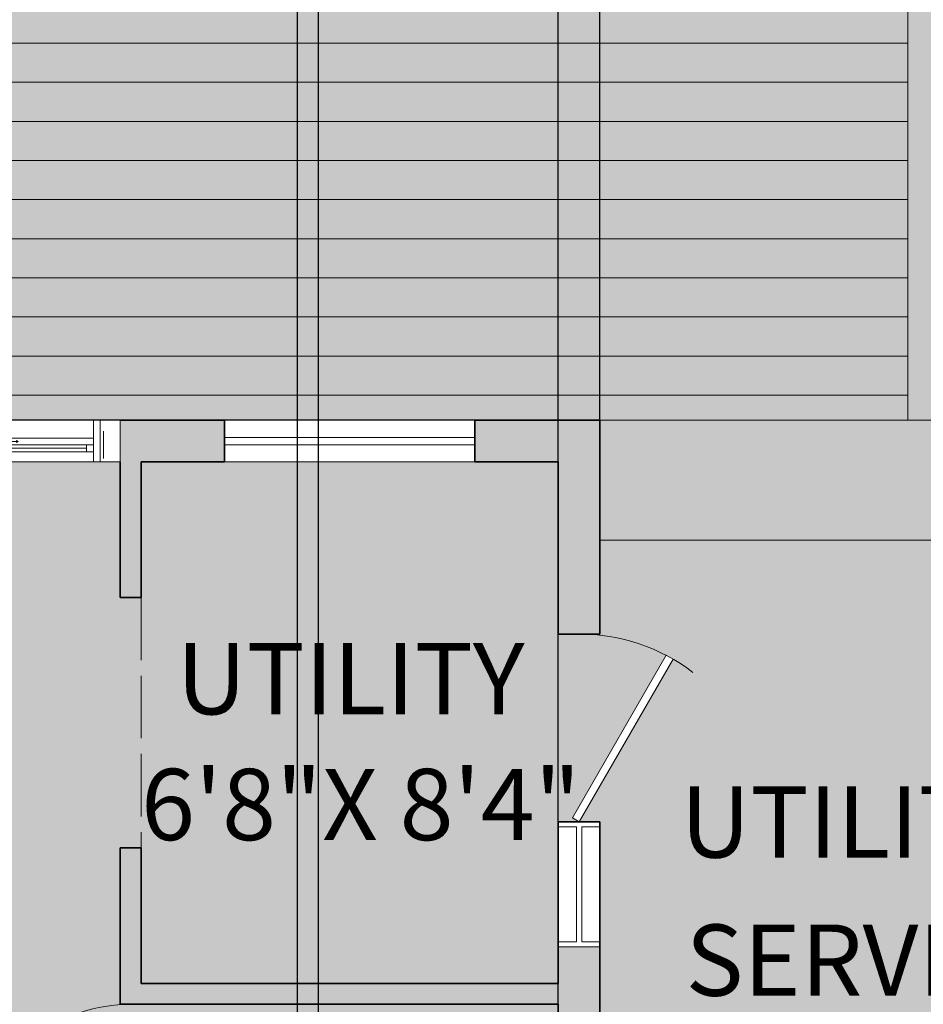
# Model space of a CAD drawing. Units: inches. Extents: x 1704 to 6393, y -157 to 1172.
# Tile 90 of 122: x 2494 to 2667, y 783 to 972. Entities that reach past the tile are written whole.
import ezdxf

# ---------------------------------------------------------------- set-up
doc = ezdxf.new("R2010")
doc.units = ezdxf.units.IN
doc.header["$MEASUREMENT"] = 0
doc.linetypes.add('ACAD_ISO02W100', pattern=[15, 12, -3])
for name, color, linetype, lineweight in [('A-ANNO-DIMS', 7, 'Continuous', 13), ('A-AREA-IDEN', 7, 'Continuous', 18), ('A-WALL-OVHD', 8, 'ACAD_ISO02W100', 13), ('A-WALL-PATT', 7, 'Continuous', 13), ('DOORS', 160, 'Continuous', 18), ('GLASS PANEL FASADE', 4, 'Continuous', 18), ('L-DECK-PLNK-PATT', 250, 'Continuous', 13), ('L-HRDS', 8, 'Continuous', 18), ('WALLS', 7, 'Continuous', 35), ('WINDOWS', 2, 'Continuous', 18)]:
    doc.layers.add(name, color=color, linetype=linetype, lineweight=lineweight)
for name, color, linetype, lineweight, true_color in [('A-FLOR-PATT', 7, 'Continuous', 13, 0xf2f2f2), ('L-DECK-PATT', 35, 'Continuous', 13, 0xa6725b), ('L-HRDS-PATT', 9, 'Continuous', 13, 0xc5c1ba)]:
    doc.layers.add(name, color=color, linetype=linetype, lineweight=lineweight, true_color=true_color)
doc.styles.get("Standard").update_dxf_attribs({"font": 'arial.ttf'})
doc.dimstyles.get("Standard").update_dxf_attribs({"dimtxt": 6, "dimasz": 2, "dimexe": 0.18, "dimexo": 0.0625, "dimgap": 0.09, "dimtad": 0, "dimtih": 1, "dimtoh": 1, "dimdec": 1, "dimzin": 0, "dimdsep": 46, "dimlunit": 3, "dimtxsty": 'Standard', "dimblk": 'ARCHTICK', "dimcen": 0.09, "dimadec": 0, "dimazin": 0, "dimtfac": 1, "dimtdec": 1, "dimtofl": 0, "dimtmove": 0, "dimatfit": 3, "dimfxl": 1, "dimtolj": 1, "dimtzin": 0, "dimarcsym": 0})

# ---------------------------------------------------------------- blocks, each defined once
blk = doc.blocks.new('Door - Left Hung 36 in.')
blk.add_lwpolyline([(0.75, -1.3), (0, 0), (31.18, 18), (31.93, 16.7)], close=True)
blk.add_arc((0, 0), 36, 0, 37.3101)
blk = doc.blocks.new('WIN-SLIDER-48')
for p, q in [((3.83, 8), (0, 8)), ((5.13, 8), (42.87, 8)), ((44.17, 8), (48, 8)), ((3.18, 5.86), (3.18, 0.65)), ((44.82, 5.86), (44.82, 0.65)), ((6.43, 4.55), (22.7, 4.55)), ((6.43, 3.9), (22.7, 3.9)), ((24, 4.55), (42.87, 4.55)), ((25.3, 3.9), (28.1, 3.9)), ((24, 1.95), (5.13, 1.95)), ((6.43, 3.25), (22.7, 3.25)), ((22.7, 2.6), (19.9, 2.6)), ((25.3, 3.25), (41.56, 3.25)), ((25.3, 2.6), (41.56, 2.6)), ((25.3, 1.95), (41.56, 1.95)), ((3.83, 0), (0, 0)), ((5.13, 0), (42.87, 0)), ((44.17, 0), (48, 0))]:
    blk.add_line(p, q)
for points in [[(5.13, 0), (3.83, 0), (3.83, 8), (5.13, 8)], [(42.87, 0), (44.17, 0), (44.17, 8), (42.87, 8)], [(5.13, 3.25), (6.43, 3.25), (6.43, 4.55), (5.13, 4.55)], [(22.7, 3.25), (24, 3.25), (24, 4.55), (22.7, 4.55)], [(28.43, 3.9), (28.1, 4.1), (28.1, 3.71)], [(19.57, 2.6), (19.9, 2.8), (19.9, 2.41)], [(24, 1.95), (25.3, 1.95), (25.3, 3.25), (24, 3.25)], [(41.56, 1.95), (42.87, 1.95), (42.87, 3.25), (41.56, 3.25)]]:
    blk.add_lwpolyline(points, close=True)
blk = doc.blocks.new('WIN-VENT-24')
for p, q in [((0, 0), (0, 24)), ((0, 24), (8, 24)), ((0, 23), (3.5, 23)), ((3.5, 23), (3.5, 1)), ((4.5, 23), (8, 23)), ((4.5, 23), (4.5, 1)), ((8, 24), (8, 0)), ((3.5, 1), (0, 1)), ((8, 1), (4.5, 1)), ((8, 0), (0, 0))]:
    blk.add_line(p, q)
blk = doc.blocks.new('_ArchTick')
at = {"color": 0, "linetype": 'ByBlock', "const_width": 0.15}
blk.add_lwpolyline([(-0.5, -0.5), (0.5, 0.5)], dxfattribs=at)
blk = doc.blocks.new('*D92')
at = {"layer": 'A-ANNO-DIMS', "color": 0, "lineweight": -2, "transparency": 16777216}
for p, q in [((2073.35, 895.28), (2073.35, 1105.29)), ((2073.35, 1105.11), (2332.66, 1105.11)), ((2605.35, 1105.11), (2346.04, 1105.11)), ((2605.35, 895.28), (2605.35, 1105.29))]:
    blk.add_line(p, q, dxfattribs=at)
at = {"layer": 'Defpoints', "color": 0, "lineweight": -3, "transparency": 16777216}
for p in [(2605.35, 1105.11), (2073.35, 895.21), (2605.35, 895.21)]:
    blk.add_point(p, dxfattribs=at)
at = {"layer": 'A-ANNO-DIMS', "color": 0, "lineweight": -2, "transparency": 16777216, "xscale": 2, "yscale": 2, "zscale": 2, "rotation": 180}
blk.add_blockref('_ArchTick', (2073.35, 1105.11), dxfattribs=at)
at = {"layer": 'A-ANNO-DIMS', "color": 0, "lineweight": -2, "transparency": 16777216, "xscale": 2, "yscale": 2, "zscale": 2}
blk.add_blockref('_ArchTick', (2605.35, 1105.11), dxfattribs=at)
at = {"layer": 'A-ANNO-DIMS', "color": 0, "transparency": 16777216, "insert": (2339.35, 1105.11), "char_height": 6, "attachment_point": 5}
blk.add_mtext('\\A1;532', dxfattribs=at)
blk = doc.blocks.new('*D93')
at = {"layer": 'A-ANNO-DIMS', "color": 0, "lineweight": -2, "transparency": 16777216}
for p, q in [((2605.29, 895.21), (1829.7, 895.21)), ((1829.88, 895.21), (1829.88, 495.87)), ((1829.88, 90.21), (1829.88, 489.56)), ((2605.29, 90.21), (1829.7, 90.21))]:
    blk.add_line(p, q, dxfattribs=at)
at = {"layer": 'Defpoints', "color": 0, "lineweight": -3, "transparency": 16777216}
for p in [(2605.35, 895.21), (1829.88, 90.21), (2605.35, 90.21)]:
    blk.add_point(p, dxfattribs=at)
at = {"layer": 'A-ANNO-DIMS', "color": 0, "lineweight": -2, "transparency": 16777216, "xscale": 2, "yscale": 2, "zscale": 2}
for p, rotation in [((1829.88, 895.21), 90), ((1829.88, 90.21), 270)]:
    blk.add_blockref('_ArchTick', p, dxfattribs=dict(at, rotation=rotation))
at = {"layer": 'A-ANNO-DIMS', "color": 0, "transparency": 16777216, "insert": (1829.88, 492.71), "char_height": 6, "attachment_point": 5}
blk.add_mtext('\\A1;805', dxfattribs=at)
blk = doc.blocks.new('*D95')
at = {"layer": 'A-ANNO-DIMS', "color": 0, "lineweight": -2, "transparency": 16777216}
for p, q in [((2605.35, 895.28), (2605.35, 1105.29)), ((2605.35, 1105.11), (2657.91, 1105.11)), ((2723.35, 1105.11), (2670.79, 1105.11)), ((2723.35, 895.28), (2723.35, 1105.29))]:
    blk.add_line(p, q, dxfattribs=at)
at = {"layer": 'Defpoints', "color": 0, "lineweight": -3, "transparency": 16777216}
for p in [(2723.35, 1105.11), (2605.35, 895.21), (2723.35, 895.21)]:
    blk.add_point(p, dxfattribs=at)
at = {"layer": 'A-ANNO-DIMS', "color": 0, "lineweight": -2, "transparency": 16777216, "xscale": 2, "yscale": 2, "zscale": 2, "rotation": 180}
blk.add_blockref('_ArchTick', (2605.35, 1105.11), dxfattribs=at)
at = {"layer": 'A-ANNO-DIMS', "color": 0, "lineweight": -2, "transparency": 16777216, "xscale": 2, "yscale": 2, "zscale": 2}
blk.add_blockref('_ArchTick', (2723.35, 1105.11), dxfattribs=at)
at = {"layer": 'A-ANNO-DIMS', "color": 0, "transparency": 16777216, "insert": (2664.35, 1105.11), "char_height": 6, "attachment_point": 5}
blk.add_mtext('\\A1;118', dxfattribs=at)
blk = doc.blocks.new('*D102')
at = {"layer": 'A-ANNO-DIMS', "color": 0, "lineweight": -2, "transparency": 16777216}
for p, q in [((2367.74, 711.28), (2367.74, 1105.29)), ((2367.74, 1105.11), (2447.61, 1105.11)), ((2547.35, 1105.11), (2467.47, 1105.11)), ((2547.35, 711.28), (2547.35, 1105.29))]:
    blk.add_line(p, q, dxfattribs=at)
at = {"layer": 'Defpoints', "color": 0, "lineweight": -3, "transparency": 16777216}
for p in [(2547.35, 1105.11), (2367.74, 711.21), (2547.35, 711.21)]:
    blk.add_point(p, dxfattribs=at)
at = {"layer": 'A-ANNO-DIMS', "color": 0, "lineweight": -2, "transparency": 16777216, "xscale": 2, "yscale": 2, "zscale": 2, "rotation": 180}
blk.add_blockref('_ArchTick', (2367.74, 1105.11), dxfattribs=at)
at = {"layer": 'A-ANNO-DIMS', "color": 0, "lineweight": -2, "transparency": 16777216, "xscale": 2, "yscale": 2, "zscale": 2}
blk.add_blockref('_ArchTick', (2547.35, 1105.11), dxfattribs=at)
at = {"layer": 'A-ANNO-DIMS', "color": 0, "transparency": 16777216, "insert": (2457.54, 1105.11), "char_height": 6, "attachment_point": 5}
blk.add_mtext('\\A1;179.6', dxfattribs=at)
blk = doc.blocks.new('*D103')
at = {"layer": 'A-ANNO-DIMS', "color": 0, "lineweight": -2, "transparency": 16777216}
for p, q in [((2551.35, 711.28), (2551.35, 1105.29)), ((2551.35, 1105.11), (2569.84, 1105.11)), ((2597.35, 1105.11), (2578.85, 1105.11)), ((2597.35, 711.28), (2597.35, 1105.29))]:
    blk.add_line(p, q, dxfattribs=at)
at = {"layer": 'Defpoints', "color": 0, "lineweight": -3, "transparency": 16777216}
for p in [(2597.35, 1105.11), (2551.35, 711.21), (2597.35, 711.21)]:
    blk.add_point(p, dxfattribs=at)
at = {"layer": 'A-ANNO-DIMS', "color": 0, "lineweight": -2, "transparency": 16777216, "xscale": 2, "yscale": 2, "zscale": 2, "rotation": 180}
blk.add_blockref('_ArchTick', (2551.35, 1105.11), dxfattribs=at)
at = {"layer": 'A-ANNO-DIMS', "color": 0, "lineweight": -2, "transparency": 16777216, "xscale": 2, "yscale": 2, "zscale": 2}
blk.add_blockref('_ArchTick', (2597.35, 1105.11), dxfattribs=at)
at = {"layer": 'A-ANNO-DIMS', "color": 0, "transparency": 16777216, "insert": (2574.35, 1105.11), "char_height": 6, "attachment_point": 5}
blk.add_mtext('\\A1;46', dxfattribs=at)

msp = doc.modelspace()

# ---------------------------------------------------------------- hatches: boundary and pattern name
at = {"layer": 'A-FLOR-PATT', "transparency": 33554528}
h = msp.add_hatch(color=256, dxfattribs=at)
h.dxf.hatch_style = 1
h.paths.add_polyline_path([(2517.349, 861.213), (2513.349, 861.213), (2513.349, 887.213), (2509.516, 887.213), (2508.215, 887.213), (2470.482, 887.213), (2469.181, 887.213), (2465.349, 887.213), (2333.349, 887.213), (2333.349, 863.213), (2325.349, 863.213), (2325.349, 763.213), (2365.349, 763.213), (2365.349, 719.213), (2513.349, 719.213), (2513.349, 753.213), (2515.349, 753.213), (2500.349, 779.194), (2501.431, 779.819), (2501.444, 779.796, -0.1041754), (2513.349, 783.146), (2513.349, 813.213), (2517.349, 813.213)])
h.paths.add_polyline_path([(2597.349, 818.213), (2601.349, 818.213), (2600.05, 818.963), (2618.034, 850.113, 0.1210664), (2601.349, 854.213), (2597.349, 854.213), (2597.349, 887.213), (2581.349, 887.213), (2533.349, 887.213), (2517.349, 887.213), (2517.349, 861.213), (2517.349, 813.213), (2517.349, 787.213), (2597.349, 787.213)])
h.paths.add_polyline_path([(2597.349, 783.213), (2517.349, 783.213), (2515.349, 783.213, 0.1210664), (2501.444, 779.796), (2516.792, 753.213), (2517.349, 753.213), (2517.349, 719.213), (2597.349, 719.213)])
at = {"layer": 'A-WALL-PATT', "transparency": 33554643}
h = msp.add_hatch(color=256, dxfattribs=at)
h.dxf.hatch_style = 1
h.paths.add_polyline_path([(2167.349, 895.213), (2073.349, 895.213), (2073.349, 887.213), (2081.349, 887.213), (2167.349, 887.213)])
h.paths.add_polyline_path([(2465.349, 895.213), (2273.349, 895.213), (2273.349, 903.213), (2263.349, 903.213), (2263.349, 895.213), (2263.349, 887.213), (2325.349, 887.213), (2325.349, 863.213), (2333.349, 863.213), (2333.349, 887.213), (2465.349, 887.213)])
h.paths.add_polyline_path([(2533.349, 895.213), (2513.349, 895.213), (2513.349, 887.213), (2513.349, 861.213), (2517.349, 861.213), (2517.349, 887.213), (2533.349, 887.213)])
h.paths.add_polyline_path([(2605.349, 895.213), (2581.349, 895.213), (2581.349, 887.213), (2597.349, 887.213), (2597.349, 854.213), (2605.349, 854.213)])
h.paths.add_polyline_path([(2605.349, 752.213), (2629.349, 752.213), (2629.349, 716.213), (2605.349, 716.213), (2605.349, 712.213), (2719.349, 712.213), (2719.349, 716.213), (2631.349, 716.213), (2631.349, 754.213), (2605.349, 754.213), (2605.349, 794.213), (2597.349, 794.213), (2597.349, 787.213), (2517.349, 787.213), (2517.349, 813.213), (2513.349, 813.213), (2513.349, 783.213), (2517.349, 783.213), (2597.349, 783.213), (2597.349, 719.213), (2517.349, 719.213), (2517.349, 753.213), (2513.349, 753.213), (2513.349, 719.213), (2365.349, 719.213), (2365.349, 763.213), (2325.349, 763.213), (2325.349, 755.213), (2357.349, 755.213), (2357.349, 719.213), (2325.349, 719.213), (2325.349, 711.213), (2547.349, 711.213), (2547.349, 615.213), (2449.349, 615.213), (2449.349, 607.213), (2514.349, 607.213), (2514.349, 546.213), (2439.349, 546.213), (2425.349, 546.213), (2425.349, 607.213), (2425.349, 615.213), (2350.349, 615.213), (2350.349, 589.713), (2358.349, 589.713), (2358.349, 610.213), (2420.349, 610.213), (2420.349, 545.213), (2358.349, 545.213), (2358.349, 565.713), (2350.349, 565.713), (2350.349, 538.213), (2469.349, 538.213), (2469.349, 459.213), (2469.349, 372.213), (2423.349, 372.213), (2423.349, 364.213), (2473.349, 364.213), (2473.349, 318.213), (2477.349, 318.213), (2477.349, 364.213), (2547.349, 364.213), (2547.349, 352.213), (2549.349, 352.213), (2549.349, 364.213), (2597.349, 364.213), (2597.349, 328.213), (2549.349, 328.213), (2547.349, 328.213), (2547.349, 326.213), (2549.349, 326.213), (2597.349, 326.213), (2605.349, 326.213), (2605.349, 377.057), (2597.349, 377.057), (2597.349, 372.213), (2477.349, 372.213), (2477.349, 451.213), (2597.349, 451.213), (2605.349, 451.213), (2605.349, 459.213), (2597.349, 459.213), (2477.349, 459.213), (2477.349, 538.213), (2597.349, 538.213), (2597.349, 495.213), (2605.349, 495.213), (2605.349, 512.213), (2631.349, 512.213), (2631.349, 568.213), (2605.349, 568.213), (2605.349, 577.213), (2597.349, 577.213), (2597.349, 542.213), (2518.349, 542.213), (2518.349, 607.213), (2532.349, 607.213), (2605.349, 607.213), (2605.349, 615.213), (2597.349, 615.213), (2551.349, 615.213), (2551.349, 711.213), (2597.349, 711.213), (2597.349, 645.213), (2605.349, 645.213), (2605.349, 712.213), (2605.349, 716.213)])
h.paths.add_polyline_path([(2605.349, 566.213), (2629.349, 566.213), (2629.349, 514.213), (2605.349, 514.213)], flags=16)
h.paths.add_polyline_path([(2381.349, 372.213), (2349.349, 372.213), (2349.349, 202.213), (2337.349, 202.213), (2337.349, 194.213), (2349.349, 194.213), (2349.349, 90.213), (2349.349, 72.213), (2357.349, 72.213), (2357.349, 90.213), (2381.349, 90.213), (2381.349, 98.213), (2357.349, 98.213), (2357.349, 266.213), (2381.349, 266.213), (2381.349, 270.213), (2353.349, 270.213), (2353.349, 364.213), (2381.349, 364.213)])
h.paths.add_polyline_path([(2605.349, 302.213), (2597.349, 302.213), (2597.349, 270.213), (2477.349, 270.213), (2477.349, 294.213), (2473.349, 294.213), (2473.349, 270.213), (2423.349, 270.213), (2423.349, 266.213), (2597.349, 266.213), (2597.349, 218.213), (2605.349, 218.213)])
h.paths.add_polyline_path([(2605.349, 146.213), (2597.349, 146.213), (2597.349, 98.213), (2429.349, 98.213), (2429.349, 90.213), (2597.349, 90.213), (2597.349, 72.213), (2605.349, 72.213), (2605.349, 90.213)])
h.paths.add_polyline_path([(2225.349, 202.213), (2049.349, 202.213), (2049.349, 194.213), (2225.349, 194.213)])
h.paths.add_polyline_path([(2289.349, 202.213), (2277.349, 202.213), (2273.349, 202.213), (2269.516, 202.213), (2269.516, 194.213), (2273.349, 194.213), (2277.349, 194.213), (2289.349, 194.213)])
h.paths.add_polyline_path([(2273.349, 372.213), (2029.19, 372.213), (2029.19, 364.213), (2273.349, 364.213)])
h.paths.add_polyline_path([(2277.349, 545.213), (2213.349, 545.213), (2213.349, 573.213), (2205.349, 573.213), (2177.349, 573.213), (2177.349, 545.213), (2073.349, 545.213), (2073.349, 538.213), (2081.349, 538.213), (2277.349, 538.213)])
h.paths.add_polyline_path([(2181.349, 545.213), (2181.349, 569.213), (2205.349, 569.213), (2205.349, 545.213)], flags=16)
h.paths.add_polyline_path([(2277.349, 719.213), (2081.349, 719.213), (2073.349, 719.213), (2073.349, 711.213), (2154.575, 711.213), (2205.349, 711.213), (2205.349, 687.213), (2205.349, 629.213), (2213.349, 629.213), (2273.349, 629.213), (2273.349, 631.213), (2207.349, 631.213), (2207.349, 707.213), (2231.349, 707.213), (2231.349, 709.213), (2207.349, 709.213), (2207.349, 711.213), (2277.349, 711.213)])
at = {"layer": 'L-DECK-PATT', "transparency": 33554544}
h = msp.add_hatch(color=256, dxfattribs=at)
h.dxf.hatch_style = 1
h.paths.add_polyline_path([(2329.589, 1033.213), (2065.589, 1033.213), (2065.589, 895.213), (2167.349, 895.213), (2263.349, 895.213), (2263.349, 903.213), (2273.349, 903.213), (2273.349, 895.213), (2329.589, 895.213)])
h.paths.add_polyline_path([(2664.349, 1033.213), (2333.589, 1033.213), (2333.589, 895.213), (2465.349, 895.213), (2469.181, 895.213), (2470.482, 895.213), (2508.215, 895.213), (2509.516, 895.213), (2513.349, 895.213), (2533.349, 895.213), (2581.349, 895.213), (2605.349, 895.213), (2664.349, 895.213)])
h.paths.add_polyline_path([(2333.589, 1033.213), (2329.589, 1033.213), (2329.589, 895.213), (2333.589, 895.213)])
at = {"layer": 'L-DECK-PLNK-PATT'}
h = msp.add_hatch(dxfattribs=at)
h.set_pattern_fill('LINE', color=256, scale=60)
h.paths.add_polyline_path([(2329.589, 1033.213), (2065.589, 1033.213), (2065.589, 895.213), (2167.349, 895.213), (2263.349, 895.213), (2263.349, 903.213), (2273.349, 903.213), (2273.349, 895.213), (2329.589, 895.213)])
h.paths.add_polyline_path([(2664.349, 1033.213), (2333.589, 1033.213), (2333.589, 895.213), (2465.349, 895.213), (2469.181, 895.213), (2470.482, 895.213), (2508.215, 895.213), (2509.516, 895.213), (2513.349, 895.213), (2533.349, 895.213), (2581.349, 895.213), (2605.349, 895.213), (2664.349, 895.213)])
h.paths.add_polyline_path([(2333.589, 1033.213), (2329.589, 1033.213), (2329.589, 895.213), (2333.589, 895.213)])
at = {"layer": 'L-HRDS-PATT', "transparency": 33554661}
h = msp.add_hatch(color=256, dxfattribs=at)
h.dxf.hatch_style = 1
h.paths.add_polyline_path([(2719.349, 1033.213), (2664.349, 1033.213), (2664.349, 895.213), (2719.349, 895.213)])
h.paths.add_polyline_path([(2719.349, 895.213), (2664.349, 895.213), (2605.349, 895.213), (2605.349, 872.213), (2719.349, 872.213)])
h.paths.add_polyline_path([(2719.349, 872.213), (2605.349, 872.213), (2605.349, 854.213), (2601.349, 854.213, -0.1210664), (2618.034, 850.113), (2618.05, 850.14), (2619.349, 849.39), (2601.349, 818.213), (2605.349, 818.213), (2605.349, 794.213), (2605.349, 754.213), (2631.349, 754.213), (2631.349, 716.213), (2719.349, 716.213)])

# ---------------------------------------------------------------- linework, layer by layer
at = {"layer": 'A-WALL-OVHD'}
msp.add_line((2517.349, 861.213), (2517.349, 813.213), dxfattribs=at)
at = {"layer": 'GLASS PANEL FASADE'}
for p, q in [((2533.349, 891.913), (2581.349, 891.913)), ((2533.349, 890.513), (2581.349, 890.513))]:
    msp.add_line(p, q, dxfattribs=at)
msp.add_lwpolyline([(2533.349, 887.213), (2533.349, 895.213), (2581.349, 895.213), (2581.349, 887.213)], close=True, dxfattribs=at)
at = {"layer": 'L-HRDS'}
for p, q in [((2664.349, 895.213), (2664.349, 1033.213)), ((2605.349, 895.213), (2723.349, 895.213)), ((2605.349, 872.213), (2723.349, 872.213))]:
    msp.add_line(p, q, dxfattribs=at)
at = {"layer": 'WALLS'}
for p, q in [((2533.349, 895.213), (2513.349, 895.213)), ((2533.349, 887.213), (2533.349, 895.213)), ((2605.349, 895.213), (2581.349, 895.213)), ((2581.349, 887.213), (2581.349, 895.213)), ((2605.349, 854.213), (2605.349, 895.213)), ((2513.349, 861.213), (2513.349, 887.213)), ((2533.349, 887.213), (2517.349, 887.213)), ((2517.349, 861.213), (2517.349, 887.213)), ((2597.349, 887.213), (2581.349, 887.213)), ((2597.349, 854.213), (2597.349, 887.213)), ((2517.349, 861.213), (2513.349, 861.213)), ((2597.349, 854.213), (2605.349, 854.213)), ((2597.349, 787.213), (2597.349, 818.213)), ((2597.349, 818.213), (2605.349, 818.213)), ((2605.349, 754.213), (2605.349, 818.213)), ((2517.349, 813.213), (2513.349, 813.213)), ((2513.349, 783.213), (2513.349, 813.213)), ((2517.349, 787.213), (2517.349, 813.213)), ((2597.349, 787.213), (2517.349, 787.213)), ((2517.349, 783.213), (2513.349, 783.213)), ((2597.349, 783.213), (2517.349, 783.213)), ((2597.349, 719.213), (2597.349, 783.213))]:
    msp.add_line(p, q, dxfattribs=at)
at = {"layer": 'WINDOWS'}
msp.add_line((2513.349, 887.213), (2513.349, 895.213), dxfattribs=at)

# ---------------------------------------------------------------- block references
at = {"layer": 'DOORS', "xscale": -1, "rotation": 270}
msp.add_blockref('Door - Left Hung 36 in.', (2601.349, 818.213), dxfattribs=at)
at = {"layer": 'DOORS', "xscale": 0.8333333333333333, "yscale": 0.8333333333333333, "zscale": 0.8333333333333333, "rotation": 90.00000000000003}
msp.add_blockref('Door - Left Hung 36 in.', (2515.349, 753.213), dxfattribs=at)
at = {"layer": 'WINDOWS'}
for name, p in [('WIN-SLIDER-48', (2465.349, 887.213)), ('WIN-VENT-24', (2597.349, 794.213))]:
    msp.add_blockref(name, p, dxfattribs=at)

# ---------------------------------------------------------------- texts
at = {"layer": 'A-ANNO-DIMS'}
msp.add_text('6\'8"X 8\'4"', height=13.6672, dxfattribs=at).set_placement((2517.349, 814.689))
at = {"layer": 'A-AREA-IDEN'}
for s, p in [('UTILITY', (2524.147, 838.811)), ('UTILITY', (2620.76, 811.34)), ('SERVICE', (2621.754, 784.847))]:
    msp.add_text(s, height=13.6672, dxfattribs=at).set_placement(p)

# ---------------------------------------------------------------- dimensions: what is measured, and where the dimension line sits
at = {"layer": 'A-ANNO-DIMS'}
for base, p1, p2, override, picture, middle in [((2605.349, 1105.107), (2073.349, 895.213), (2605.349, 895.213), {"dimdec": 0, "dimlfac": 1, "dimrnd": 0, "dimzin": 0, "dimdsep": 46, "dimlunit": 2}, '*D92', (2339.349, 1105.107)), ((2547.349, 1105.107), (2367.738, 711.213), (2547.349, 711.213), {"dimdec": 1, "dimlfac": 1, "dimrnd": 0, "dimzin": 0, "dimdsep": 46, "dimlunit": 2}, '*D102', (2457.543, 1105.107)), ((2597.349, 1105.107), (2551.349, 711.213), (2597.349, 711.213), {"dimdec": 0, "dimlfac": 1, "dimrnd": 0, "dimzin": 0, "dimdsep": 46, "dimlunit": 2}, '*D103', (2574.349, 1105.107)), ((2723.349, 1105.107), (2605.349, 895.213), (2723.349, 895.213), {"dimdec": 0, "dimlfac": 1, "dimrnd": 0, "dimzin": 0, "dimdsep": 46, "dimlunit": 2}, '*D95', (2664.349, 1105.107))]:
    dim = msp.add_linear_dim(base=base, p1=p1, p2=p2, dimstyle='Standard', override=override, dxfattribs=at)
    dim.commit()
    dim.dimension.update_dxf_attribs({"geometry": picture, "text_midpoint": middle})
dim = msp.add_linear_dim(base=(1829.878, 90.213), p1=(2605.349, 895.213), p2=(2605.349, 90.213), angle=90, dimstyle='Standard', override={"dimdec": 0, "dimlfac": 1, "dimrnd": 0, "dimzin": 0, "dimdsep": 46, "dimlunit": 2}, dxfattribs=at)
dim.commit()
dim.dimension.update_dxf_attribs({"geometry": '*D93', "text_midpoint": (1829.878, 492.713)})

doc.saveas('drawing.dxf')
